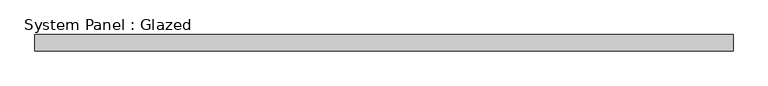
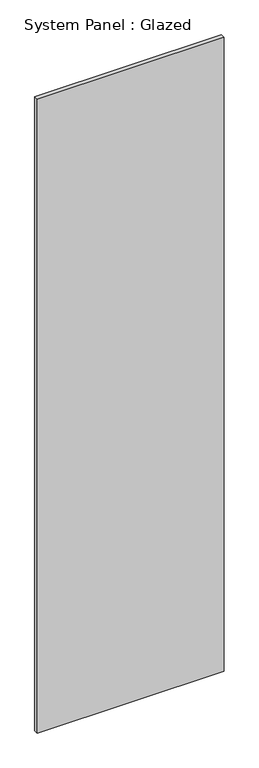
"""IFC4 building model written with IfcOpenShell, lengths in millimetres: plate geometry, System Panel : Glazed."""

from ifc_helpers import new_model, si_unit, origin, origin_with_axes, place, context, project, spatial, polyline, outline, extrude, source, transform, mapped, element, save


def system_panel_glazed_cfc6ab68(model_context):
    return source(origin(), model_context, "Body", "SweptSolid", [
        extrude(outline(polyline([(546.1, 19.05), (-546.1, 19.05), (-546.1, 44.45), (546.1, 44.45), (546.1, 19.05)])), origin_with_axes(), (0.0, 0.0, 1.0), 3915.8994026),
    ])


if __name__ == "__main__":
    model = new_model("IFC4")
    model_context = context("Model", 3, world=origin())
    ifc_project = project(units=[si_unit("LENGTHUNIT", "METRE", prefix="MILLI")], contexts=[model_context])
    site = spatial("IfcSite", under=ifc_project)
    building = spatial("IfcBuilding", under=site)
    placement = place(None, origin())
    system_panel_glazed_shape = system_panel_glazed_cfc6ab68(model_context)
    element("IfcPlate", 1, ObjectType="System Panel : Glazed", at=placement, inside=building, context=model_context, shape_type="MappedRepresentation", body=[
        mapped(system_panel_glazed_shape, transform((0.0, 0.0, 0.0), x_axis=(1.0, 0.0, 0.0), y_axis=(0.0, 1.0, 0.0), z_axis=(0.0, 0.0, 1.0))),
    ])
    save(model, "model.ifc")

# Revit data of these elements
# Type "System Panel : Glazed"
#   Construction Type Id = "GSP4R"
#   Analytic Construction = "1/8 in Pilkington single glazing"
#   Visual Light Transmittance = 0.9
#   Solar Heat Gain Coefficient = 0.86
#   Heat Transfer Coefficient (U) = 1.18115 BTU/(h·ft²·°F)
#   Define Thermal Properties by = 1
# Element 1 (IfcPlate, "System Panel : Glazed")
#   Materials on its faces: "Glass"
# Materials
#   "Glass": class "Glass", colour RGB 0 128 192, transparency 0.75, Description = "Soda Lime Glass", Cost = 0
